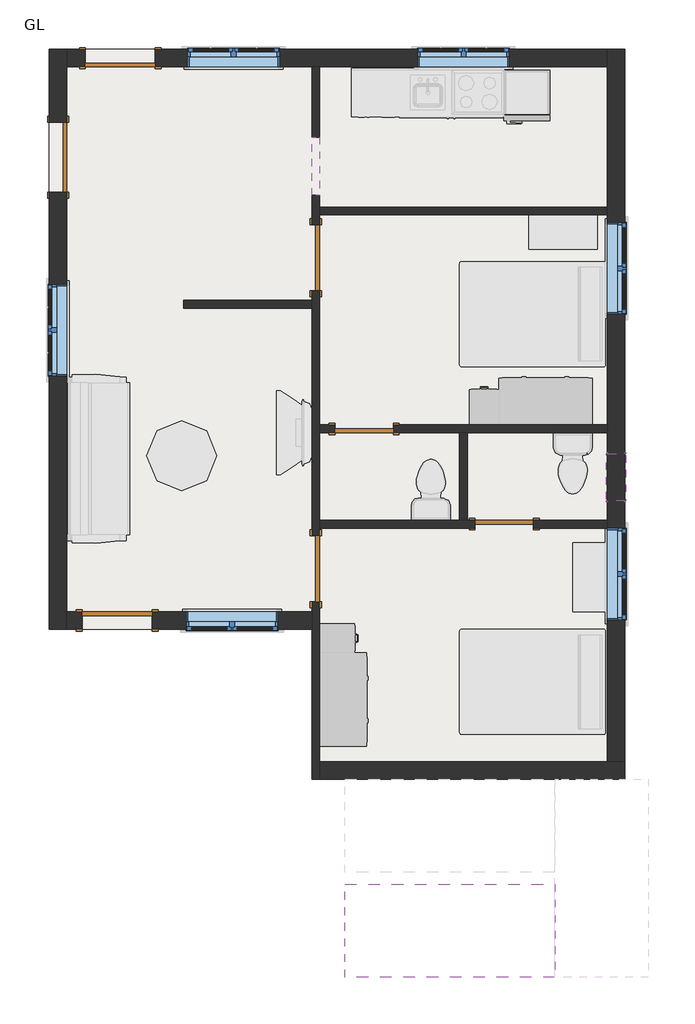
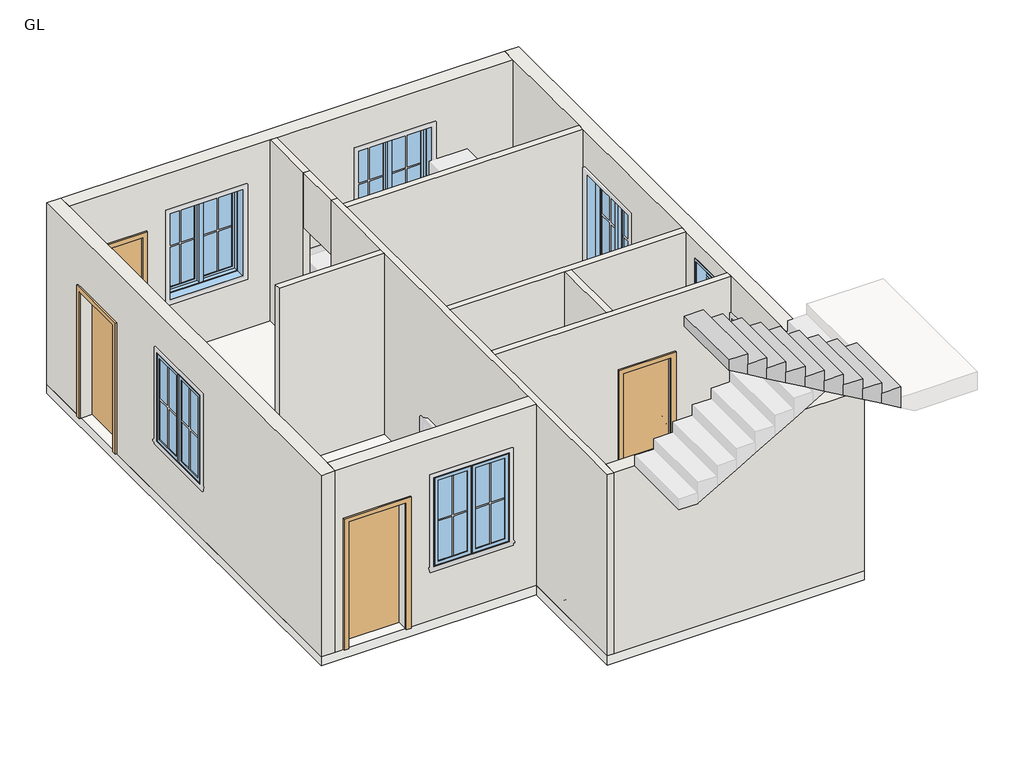
# One storey, part 1 of 2: 13 walls, 7 doors, 7 windows, 1 slab, 1 stair flight.
"""IFC4 building model written with IfcOpenShell, lengths in millimetres."""

from ifc_helpers import new_model, si_unit, frame, origin, origin_with_axes, place, context, project, spatial, polyline, outline, extrude, faceted_brep, transform, mapped, element, save
from components import m_single_flush_0762_x_2032mm_63ada305, m_single_flush_0762_x_2032mm_debabc81, m_single_flush_0864_x_2032mm_c62421c0, m_single_flush_0915_x_2134mm_43602619, m_single_flush_0915_x_2134mm_1ddf3370, m_window_casement_double_1200_x_1500mm_04159c99, window_f2d8fef0

model = new_model("IFC4")

# Units and contexts
model_context = context("Model", 3, world=origin())
ifc_project = project(units=[si_unit("LENGTHUNIT", "METRE", prefix="MILLI")], contexts=[model_context])

# Site, building, storey
site = spatial("IfcSite", under=ifc_project)
building = spatial("IfcBuilding", under=site)
storey = spatial("IfcBuildingStorey", under=building, Name="GL", Elevation=0.0)

# Doors
placement = place(None, origin())
m_single_flush_0762_x_2032mm_shape = m_single_flush_0762_x_2032mm_63ada305(model_context)
element("IfcDoor", 1, ObjectType="M_Single-Flush : 0762 x 2032mm", at=placement, inside=storey, context=model_context, shape_type="MappedRepresentation", body=[
    mapped(m_single_flush_0762_x_2032mm_shape, transform((2297.1455952, -1088.4648653, 0.0), x_axis=(-1.0, 0.0, 0.0), y_axis=(0.0, -1.0, 0.0), z_axis=(0.0, 0.0, 1.0))),
])
m_single_flush_0762_x_2032mm_2_shape = m_single_flush_0762_x_2032mm_debabc81(model_context)
element("IfcDoor", 2, ObjectType="M_Single-Flush : 0762 x 2032mm", at=placement, inside=storey, context=model_context, shape_type="MappedRepresentation", body=[
    mapped(m_single_flush_0762_x_2032mm_2_shape, transform((466.7455952, 156.1351347, 0.0), x_axis=(-1.0, 0.0, 0.0), y_axis=(0.0, -1.0, 0.0), z_axis=(0.0, 0.0, 1.0))),
])
m_single_flush_0864_x_2032mm_shape = m_single_flush_0864_x_2032mm_c62421c0(model_context)
element("IfcDoor", 3, ObjectType="M_Single-Flush : 0864 x 2032mm", at=placement, inside=storey, context=model_context, shape_type="MappedRepresentation", body=[
    mapped(m_single_flush_0864_x_2032mm_shape, transform((-165.0544048, 2391.3351347, 0.0), x_axis=(0.0, 1.0, 0.0), y_axis=(-1.0, 0.0, 0.0), z_axis=(0.0, 0.0, 1.0))),
])
element("IfcDoor", 4, ObjectType="M_Single-Flush : 0864 x 2032mm", at=placement, inside=storey, context=model_context, shape_type="MappedRepresentation", body=[
    mapped(m_single_flush_0864_x_2032mm_shape, transform((-165.0544048, -1671.2648653, 0.0), x_axis=(0.0, 1.0, 0.0), y_axis=(-1.0, 0.0, 0.0), z_axis=(0.0, 0.0, 1.0))),
])
m_single_flush_0915_x_2134mm_shape = m_single_flush_0915_x_2134mm_43602619(model_context)
element("IfcDoor", 5, ObjectType="M_Single-Flush : 0915 x 2134mm", at=placement, inside=storey, context=model_context, shape_type="MappedRepresentation", body=[
    mapped(m_single_flush_0915_x_2134mm_shape, transform((-2758.7544048, -2345.7648653, 0.0), x_axis=(-1.0, 0.0, 0.0), y_axis=(0.0, -1.0, 0.0), z_axis=(0.0, 0.0, 1.0))),
])
element("IfcDoor", 6, ObjectType="M_Single-Flush : 0915 x 2134mm", at=placement, inside=storey, context=model_context, shape_type="MappedRepresentation", body=[
    mapped(m_single_flush_0915_x_2134mm_shape, transform((-3530.5544048, 3703.0351347, 0.0), x_axis=(0.0, 1.0, 0.0), y_axis=(-1.0, 0.0, 0.0), z_axis=(0.0, 0.0, 1.0))),
])
m_single_flush_0915_x_2134mm_2_shape = m_single_flush_0915_x_2134mm_1ddf3370(model_context)
element("IfcDoor", 7, ObjectType="M_Single-Flush : 0915 x 2134mm", at=placement, inside=storey, context=model_context, shape_type="MappedRepresentation", body=[
    mapped(m_single_flush_0915_x_2134mm_2_shape, transform((-2718.7544048, 4994.8351347, 0.0), x_axis=(-1.0, 0.0, 0.0), y_axis=(0.0, -1.0, 0.0), z_axis=(0.0, 0.0, 1.0))),
])

# Slab
element("IfcSlab", 8, ObjectType="6\" floor", at=placement, inside=storey, context=model_context, shape_type="SweptSolid", body=[
    extrude(outline(polyline([(3873.5455952, 5109.1351347), (3873.5455952, -4415.8648653), (-215.8544048, -4415.8648653), (-215.8544048, -2460.0648653), (-3644.8544048, -2460.0648653), (-3644.8544048, 5109.1351347), (3873.5455952, 5109.1351347)])), frame((0.0, 0.0, -152.4), z_axis=(0.0, 0.0, 1.0), x_axis=(1.0, 0.0, 0.0)), (0.0, 0.0, 1.0), 152.4),
])

# Stair flight
element("IfcStairFlight", 9, ObjectType="150mm Depth", at=placement, inside=storey, context=model_context, shape_type="Brep", body=[
    faceted_brep([(2654.3455952, -7006.6648653, 4989.0947368), (2959.1455952, -7006.6648653, 4989.0947368), (2959.1455952, -5787.4648653, 4989.0947368), (2654.3455952, -5787.4648653, 4989.0947368), (2654.3455952, -7006.6648653, 4815.7697495), (2959.1455952, -7006.6648653, 4639.3065916), (2959.1455952, -7006.6648653, 4812.6315789), (2959.1455952, -5787.4648653, 4639.3065916), (2654.3455952, -5787.4648653, 4815.7697495), (2349.5455952, -7006.6648653, 5165.5578947), (2654.3455952, -7006.6648653, 5165.5578947), (2654.3455952, -5787.4648653, 5165.5578947), (2349.5455952, -5787.4648653, 5165.5578947), (2349.5455952, -7006.6648653, 4992.2329074), (2349.5455952, -5787.4648653, 4992.2329074), (2044.7455952, -7006.6648653, 5342.0210526), (2349.5455952, -7006.6648653, 5342.0210526), (2349.5455952, -5787.4648653, 5342.0210526), (2044.7455952, -5787.4648653, 5342.0210526), (2044.7455952, -7006.6648653, 5168.6960653), (2044.7455952, -5787.4648653, 5168.6960653), (1739.9455952, -7006.6648653, 5518.4842105), (2044.7455952, -7006.6648653, 5518.4842105), (2044.7455952, -5787.4648653, 5518.4842105), (1739.9455952, -5787.4648653, 5518.4842105), (1739.9455952, -7006.6648653, 5345.1592232), (1739.9455952, -5787.4648653, 5345.1592232), (1435.1455952, -7006.6648653, 5694.9473684), (1739.9455952, -7006.6648653, 5694.9473684), (1739.9455952, -5787.4648653, 5694.9473684), (1435.1455952, -5787.4648653, 5694.9473684), (1435.1455952, -7006.6648653, 5521.6223811), (1435.1455952, -5787.4648653, 5521.6223811), (1130.3455952, -7006.6648653, 5871.4105263), (1435.1455952, -7006.6648653, 5871.4105263), (1435.1455952, -5787.4648653, 5871.4105263), (1130.3455952, -5787.4648653, 5871.4105263), (1130.3455952, -7006.6648653, 5698.0855389), (1130.3455952, -5787.4648653, 5698.0855389), (825.5455952, -7006.6648653, 6047.8736842), (1130.3455952, -7006.6648653, 6047.8736842), (1130.3455952, -5787.4648653, 6047.8736842), (825.5455952, -5787.4648653, 6047.8736842), (825.5455952, -7006.6648653, 5874.5486968), (825.5455952, -5787.4648653, 5874.5486968), (520.7455952, -7006.6648653, 6224.3368421), (825.5455952, -7006.6648653, 6224.3368421), (825.5455952, -5787.4648653, 6224.3368421), (520.7455952, -5787.4648653, 6224.3368421), (520.7455952, -7006.6648653, 6051.0118547), (520.7455952, -5787.4648653, 6051.0118547), (215.9455952, -7006.6648653, 6400.8), (520.7455952, -7006.6648653, 6400.8), (520.7455952, -5787.4648653, 6400.8), (215.9455952, -5787.4648653, 6400.8), (215.9455952, -7006.6648653, 6227.4750126), (215.9455952, -5787.4648653, 6227.4750126)], [[[0, 1, 2, 3]], [[1, 0, 4, 5, 6]], [[2, 1, 6, 5, 7]], [[3, 2, 7, 8]], [[9, 10, 11, 12]], [[10, 9, 13, 4, 0]], [[11, 10, 0, 3]], [[12, 11, 3, 8, 14]], [[15, 16, 17, 18]], [[16, 15, 19, 13, 9]], [[17, 16, 9, 12]], [[18, 17, 12, 14, 20]], [[21, 22, 23, 24]], [[22, 21, 25, 19, 15]], [[23, 22, 15, 18]], [[24, 23, 18, 20, 26]], [[27, 28, 29, 30]], [[28, 27, 31, 25, 21]], [[29, 28, 21, 24]], [[30, 29, 24, 26, 32]], [[33, 34, 35, 36]], [[34, 33, 37, 31, 27]], [[35, 34, 27, 30]], [[36, 35, 30, 32, 38]], [[39, 40, 41, 42]], [[40, 39, 43, 37, 33]], [[41, 40, 33, 36]], [[42, 41, 36, 38, 44]], [[45, 46, 47, 48]], [[46, 45, 49, 43, 39]], [[47, 46, 39, 42]], [[48, 47, 42, 44, 50]], [[51, 52, 53, 54]], [[52, 51, 55, 49, 45]], [[53, 52, 45, 48]], [[54, 53, 48, 50, 56]], [[51, 54, 56, 55]], [[5, 4, 13, 19, 25, 31, 37, 43, 49, 55, 56, 50, 44, 38, 32, 26, 20, 14, 8, 7]]]),
])

# Walls
element("IfcWall", 10, ObjectType="4\" wall", at=placement, inside=storey, context=model_context, shape_type="Brep", body=[
    faceted_brep([(-215.8544048, 3204.1351347, 0.0), (-215.8544048, 2823.3351347, 0.0), (-215.8544048, 2823.3351347, 2032.0), (-215.8544048, 1959.3351347, 2032.0), (-215.8544048, 1959.3351347, 0.0), (-215.8544048, 1832.5351347, 0.0), (-215.8544048, 1730.9351347, 0.0), (-215.8544048, -1239.2648653, 0.0), (-215.8544048, -1239.2648653, 2032.0), (-215.8544048, -2103.2648653, 2032.0), (-215.8544048, -2103.2648653, 0.0), (-215.8544048, -2231.4648653, 0.0), (-215.8544048, -2460.0648653, 0.0), (-215.8544048, -4415.8648653, 0.0), (-215.8544048, -4415.8648653, 3048.0), (-215.8544048, -2460.0648653, 3048.0), (-215.8544048, -2231.4648653, 3048.0), (-215.8544048, 1730.9351347, 3048.0), (-215.8544048, 1832.5351347, 3048.0), (-215.8544048, 3204.1351347, 3048.0), (-215.8544048, 3204.1351347, 2133.6), (-114.2544048, 2823.3351347, 2032.0), (-114.2544048, 2823.3351347, 0.0), (-114.2544048, 2950.1351347, 0.0), (-114.2544048, 3051.7351347, 0.0), (-114.2544048, 3204.1351347, 0.0), (-114.2544048, 3204.1351347, 2133.6), (-114.2544048, 3204.1351347, 3048.0), (-114.2544048, 3051.7351347, 3048.0), (-114.2544048, 2950.1351347, 3048.0), (-114.2544048, 206.9351347, 3048.0), (-114.2544048, 105.3351347, 3048.0), (-114.2544048, -1037.6648653, 3048.0), (-114.2544048, -1139.2648653, 3048.0), (-114.2544048, -4187.2648653, 3048.0), (-114.2544048, -4415.8648653, 3048.0), (-114.2544048, -4415.8648653, 0.0), (-114.2544048, -4187.2648653, 0.0), (-114.2544048, -2103.2648653, 0.0), (-114.2544048, -2103.2648653, 2032.0), (-114.2544048, -1239.2648653, 2032.0), (-114.2544048, -1239.2648653, 0.0), (-114.2544048, -1139.2648653, 0.0), (-114.2544048, -1037.6648653, 0.0), (-114.2544048, 105.3351347, 0.0), (-114.2544048, 206.9351347, 0.0), (-114.2544048, 1959.3351347, 0.0), (-114.2544048, 1959.3351347, 2032.0)], [[[0, 1, 2, 3, 4, 5, 6, 7, 8, 9, 10, 11, 12, 13, 14, 15, 16, 17, 18, 19, 20]], [[21, 22, 23, 24, 25, 26, 27, 28, 29, 30, 31, 32, 33, 34, 35, 36, 37, 38, 39, 40, 41, 42, 43, 44, 45, 46, 47]], [[36, 13, 12, 11, 10, 38, 37]], [[25, 24, 23, 22, 1, 0]], [[46, 45, 44, 43, 42, 41, 7, 6, 5, 4]], [[19, 18, 17, 16, 15, 14, 35, 34, 33, 32, 31, 30, 29, 28, 27]], [[0, 20, 19, 27, 26, 25]], [[14, 13, 36, 35]], [[8, 40, 39, 9]], [[9, 39, 38, 10]], [[4, 3, 47, 46]], [[3, 2, 21, 47]], [[2, 1, 22, 21]], [[40, 8, 7, 41]]]),
])
element("IfcWall", 11, ObjectType="4\" wall", at=placement, inside=storey, context=model_context, shape_type="Brep", body=[
    faceted_brep([(-114.2544048, -1139.2648653, 0.0), (1916.1455952, -1139.2648653, 0.0), (1916.1455952, -1139.2648653, 2032.0), (2678.1455952, -1139.2648653, 2032.0), (2678.1455952, -1139.2648653, 0.0), (3644.9455952, -1139.2648653, 0.0), (3644.9455952, -1139.2648653, 900.0), (3644.9455952, -1139.2648653, 2400.0), (3644.9455952, -1139.2648653, 3048.0), (-114.2544048, -1139.2648653, 3048.0), (1916.1455952, -1037.6648653, 2032.0), (1916.1455952, -1037.6648653, 0.0), (1816.1455952, -1037.6648653, 0.0), (1714.5455952, -1037.6648653, 0.0), (-114.2544048, -1037.6648653, 0.0), (-114.2544048, -1037.6648653, 3048.0), (1714.5455952, -1037.6648653, 3048.0), (1816.1455952, -1037.6648653, 3048.0), (3644.9455952, -1037.6648653, 3048.0), (3644.9455952, -1037.6648653, 0.0), (2678.1455952, -1037.6648653, 0.0), (2678.1455952, -1037.6648653, 2032.0)], [[[0, 1, 2, 3, 4, 5, 6, 7, 8, 9]], [[10, 11, 12, 13, 14, 15, 16, 17, 18, 19, 20, 21]], [[20, 19, 5, 4]], [[14, 13, 12, 11, 1, 0]], [[9, 8, 18, 17, 16, 15]], [[8, 7, 6, 5, 19, 18]], [[0, 9, 15, 14]], [[2, 1, 11, 10]], [[3, 2, 10, 21]], [[4, 3, 21, 20]]]),
])
element("IfcWall", 12, ObjectType="4\" wall", at=placement, inside=storey, context=model_context, shape_type="Brep", body=[
    faceted_brep([(85.7455952, 206.9351347, 2032.0), (85.7455952, 206.9351347, 0.0), (-114.2544048, 206.9351347, 0.0), (-114.2544048, 206.9351347, 3048.0), (3644.9455952, 206.9351347, 3048.0), (3644.9455952, 206.9351347, 0.0), (847.7455952, 206.9351347, 0.0), (847.7455952, 206.9351347, 2032.0), (-114.2544048, 105.3351347, 0.0), (85.7455952, 105.3351347, 0.0), (85.7455952, 105.3351347, 2032.0), (847.7455952, 105.3351347, 2032.0), (847.7455952, 105.3351347, 0.0), (1714.5455952, 105.3351347, 0.0), (1816.1455952, 105.3351347, 0.0), (3644.9455952, 105.3351347, 0.0), (3644.9455952, 105.3351347, 3048.0), (1816.1455952, 105.3351347, 3048.0), (1714.5455952, 105.3351347, 3048.0), (-114.2544048, 105.3351347, 3048.0)], [[[0, 1, 2, 3, 4, 5, 6, 7]], [[8, 9, 10, 11, 12, 13, 14, 15, 16, 17, 18, 19]], [[6, 5, 15, 14, 13, 12]], [[2, 1, 9, 8]], [[4, 3, 19, 18, 17, 16]], [[5, 4, 16, 15]], [[3, 2, 8, 19]], [[10, 9, 1, 0]], [[11, 10, 0, 7]], [[12, 11, 7, 6]]]),
])
element("IfcWall", 13, ObjectType="4\" wall", at=placement, inside=storey, context=model_context, shape_type="SweptSolid", body=[
    extrude(outline(polyline([(-215.8544048, 1730.9351347), (-1892.2544048, 1730.9351347), (-1892.2544048, 1832.5351347), (-215.8544048, 1832.5351347), (-215.8544048, 1730.9351347)])), origin_with_axes(), (0.0, 0.0, 1.0), 3048.0),
])
element("IfcWall", 14, ObjectType="4\" wall", at=placement, inside=storey, context=model_context, shape_type="SweptSolid", body=[
    extrude(outline(polyline([(-114.2544048, 3051.7351347), (3644.9455952, 3051.7351347), (3644.9455952, 2950.1351347), (-114.2544048, 2950.1351347), (-114.2544048, 3051.7351347)])), origin_with_axes(), (0.0, 0.0, 1.0), 3048.0),
])
element("IfcWall", 15, ObjectType="4\" wall", at=placement, inside=storey, context=model_context, shape_type="SweptSolid", body=[
    extrude(outline(polyline([(1714.5455952, -1037.6648653), (1714.5455952, 105.3351347), (1816.1455952, 105.3351347), (1816.1455952, -1037.6648653), (1714.5455952, -1037.6648653)])), origin_with_axes(), (0.0, 0.0, 1.0), 3048.0),
])
element("IfcWall", 16, ObjectType="4\" wall", at=placement, inside=storey, context=model_context, shape_type="Brep", body=[
    faceted_brep([(-215.8544048, 4880.5351347, 0.0), (-215.8544048, 3966.1351347, 0.0), (-215.8544048, 3966.1351347, 2133.6), (-215.8544048, 3966.1351347, 3048.0), (-215.8544048, 4880.5351347, 3048.0), (-114.2544048, 4880.5351347, 0.0), (-114.2544048, 4880.5351347, 3048.0), (-114.2544048, 3966.1351347, 3048.0), (-114.2544048, 3966.1351347, 2133.6), (-114.2544048, 3966.1351347, 0.0)], [[[0, 1, 2, 3, 4]], [[5, 6, 7, 8, 9]], [[1, 0, 5, 9]], [[3, 2, 1, 9, 8, 7]], [[4, 3, 7, 6]], [[0, 4, 6, 5]]]),
])
element("IfcWall", 17, ObjectType="4\" wall", at=placement, inside=storey, context=model_context, shape_type="SweptSolid", body=[
    extrude(outline(polyline([(-215.8544048, 3204.1351347), (-215.8544048, 3966.1351347), (-114.2544048, 3966.1351347), (-114.2544048, 3204.1351347), (-215.8544048, 3204.1351347)])), frame((0.0, 0.0, 2133.6), z_axis=(0.0, 0.0, 1.0), x_axis=(1.0, 0.0, 0.0)), (0.0, 0.0, 1.0), 914.4),
])
element("IfcWall", 18, ObjectType="9\" wall", at=placement, inside=storey, context=model_context, shape_type="Brep", body=[
    faceted_brep([(-3644.8544048, 5109.1351347, 0.0), (-3644.8544048, 4160.5351347, 0.0), (-3644.8544048, 4160.5351347, 2134.0), (-3644.8544048, 3245.5351347, 2134.0), (-3644.8544048, 3245.5351347, 0.0), (-3644.8544048, -2460.0648653, 0.0), (-3644.8544048, -2460.0648653, 3048.0), (-3644.8544048, 5109.1351347, 3048.0), (-3644.8544048, 2045.5351347, 2400.0), (-3644.8544048, 845.5351347, 2400.0), (-3644.8544048, 845.5351347, 900.0), (-3644.8544048, 2045.5351347, 900.0), (-3416.2544048, 4160.5351347, 2134.0), (-3416.2544048, 4160.5351347, 0.0), (-3416.2544048, 4880.5351347, 0.0), (-3416.2544048, 5109.1351347, 0.0), (-3416.2544048, 5109.1351347, 3048.0), (-3416.2544048, 4880.5351347, 3048.0), (-3416.2544048, -2231.4648653, 3048.0), (-3416.2544048, -2460.0648653, 3048.0), (-3416.2544048, -2460.0648653, 0.0), (-3416.2544048, -2231.4648653, 0.0), (-3416.2544048, 3245.5351347, 0.0), (-3416.2544048, 3245.5351347, 2134.0), (-3416.2544048, 2045.5351347, 2400.0), (-3416.2544048, 2045.5351347, 900.0), (-3416.2544048, 845.5351347, 900.0), (-3416.2544048, 845.5351347, 2400.0)], [[[0, 1, 2, 3, 4, 5, 6, 7], [8, 9, 10, 11]], [[12, 13, 14, 15, 16, 17, 18, 19, 20, 21, 22, 23], [24, 25, 26, 27]], [[15, 14, 13, 1, 0]], [[22, 21, 20, 5, 4]], [[7, 6, 19, 18, 17, 16]], [[6, 5, 20, 19]], [[0, 7, 16, 15]], [[2, 1, 13, 12]], [[3, 2, 12, 23]], [[4, 3, 23, 22]], [[25, 24, 8, 11]], [[26, 25, 11, 10]], [[27, 26, 10, 9]], [[24, 27, 9, 8]]]),
])
element("IfcWall", 19, ObjectType="9\" wall", at=placement, inside=storey, context=model_context, shape_type="SweptSolid", body=[
    extrude(outline(polyline([(0.0, -3416.2544048), (0.0, -3216.2544048), (2134.0, -3216.2544048), (2134.0, -2301.2544048), (0.0, -2301.2544048), (0.0, -215.8544048), (3048.0, -215.8544048), (3048.0, -3416.2544048), (0.0, -3416.2544048)]), holes=[polyline([(2400.0, -1858.5544048), (2400.0, -658.5544048), (900.0, -658.5544048), (900.0, -1858.5544048), (2400.0, -1858.5544048)])]), frame((0.0, -2460.0648653, 0.0), z_axis=(0.0, 1.0, 0.0), x_axis=(0.0, 0.0, 1.0)), (0.0, 0.0, 1.0), 228.6),
])
element("IfcWall", 20, ObjectType="9\" wall", at=placement, inside=storey, context=model_context, shape_type="Brep", body=[
    faceted_brep([(-114.2544048, -4415.8648653, 0.0), (3873.5455952, -4415.8648653, 0.0), (3873.5455952, -4415.8648653, 3048.0), (-114.2544048, -4415.8648653, 3048.0), (-114.2544048, -4187.2648653, 0.0), (-114.2544048, -4187.2648653, 3048.0), (3644.9455952, -4187.2648653, 3048.0), (3873.5455952, -4187.2648653, 3048.0), (3873.5455952, -4187.2648653, 0.0), (3644.9455952, -4187.2648653, 0.0)], [[[0, 1, 2, 3]], [[4, 5, 6, 7, 8, 9]], [[1, 0, 4, 9, 8]], [[3, 2, 7, 6, 5]], [[0, 3, 5, 4]], [[2, 1, 8, 7]]]),
])
element("IfcWall", 21, ObjectType="9\" wall", at=placement, inside=storey, context=model_context, shape_type="Brep", body=[
    faceted_brep([(3873.5455952, -4187.2648653, 0.0), (3873.5455952, 5109.1351347, 0.0), (3873.5455952, 5109.1351347, 3048.0), (3873.5455952, -4187.2648653, 3048.0), (3873.5455952, 1650.1351347, 2400.0), (3873.5455952, 2850.1351347, 2400.0), (3873.5455952, 2850.1351347, 900.0), (3873.5455952, 1650.1351347, 900.0), (3873.5455952, -2339.2648653, 2400.0), (3873.5455952, -1139.2648653, 2400.0), (3873.5455952, -1139.2648653, 900.0), (3873.5455952, -2339.2648653, 900.0), (3873.5455952, -170.8898653, 2743.2), (3873.5455952, -170.8898653, 2133.6), (3873.5455952, -780.4898653, 2133.6), (3873.5455952, -780.4898653, 2743.2), (3644.9455952, -4187.2648653, 0.0), (3644.9455952, -4187.2648653, 3048.0), (3644.9455952, -1139.2648653, 3048.0), (3644.9455952, -1037.6648653, 3048.0), (3644.9455952, 105.3351347, 3048.0), (3644.9455952, 206.9351347, 3048.0), (3644.9455952, 2950.1351347, 3048.0), (3644.9455952, 3051.7351347, 3048.0), (3644.9455952, 4880.5351347, 3048.0), (3644.9455952, 5109.1351347, 3048.0), (3644.9455952, 5109.1351347, 0.0), (3644.9455952, 4880.5351347, 0.0), (3644.9455952, 3051.7351347, 0.0), (3644.9455952, 2950.1351347, 0.0), (3644.9455952, 206.9351347, 0.0), (3644.9455952, 105.3351347, 0.0), (3644.9455952, -1037.6648653, 0.0), (3644.9455952, -1139.2648653, 0.0), (3644.9455952, 1650.1351347, 2400.0), (3644.9455952, 1650.1351347, 900.0), (3644.9455952, 2850.1351347, 900.0), (3644.9455952, 2850.1351347, 2400.0), (3644.9455952, -2339.2648653, 2400.0), (3644.9455952, -2339.2648653, 900.0), (3644.9455952, -1139.2648653, 900.0), (3644.9455952, -1139.2648653, 2400.0), (3644.9455952, -170.8898653, 2743.2), (3644.9455952, -780.4898653, 2743.2), (3644.9455952, -780.4898653, 2133.6), (3644.9455952, -170.8898653, 2133.6)], [[[0, 1, 2, 3], [4, 5, 6, 7], [8, 9, 10, 11], [12, 13, 14, 15]], [[16, 17, 18, 19, 20, 21, 22, 23, 24, 25, 26, 27, 28, 29, 30, 31, 32, 33], [34, 35, 36, 37], [38, 39, 40, 41], [42, 43, 44, 45]], [[1, 0, 16, 33, 32, 31, 30, 29, 28, 27, 26]], [[3, 2, 25, 24, 23, 22, 21, 20, 19, 18, 17]], [[0, 3, 17, 16]], [[2, 1, 26, 25]], [[35, 34, 4, 7]], [[36, 35, 7, 6]], [[37, 36, 6, 5]], [[34, 37, 5, 4]], [[39, 38, 8, 11]], [[40, 39, 11, 10]], [[41, 40, 10, 9]], [[38, 41, 9, 8]], [[13, 12, 42, 45]], [[14, 13, 45, 44]], [[15, 14, 44, 43]], [[12, 15, 43, 42]]]),
])
element("IfcWall", 22, ObjectType="9\" wall", at=placement, inside=storey, context=model_context, shape_type="Brep", body=[
    faceted_brep([(-3176.2544048, 5109.1351347, 2134.0), (-3176.2544048, 5109.1351347, 0.0), (-3416.2544048, 5109.1351347, 0.0), (-3416.2544048, 5109.1351347, 3048.0), (3644.9455952, 5109.1351347, 3048.0), (3644.9455952, 5109.1351347, 0.0), (-2261.2544048, 5109.1351347, 0.0), (-2261.2544048, 5109.1351347, 2134.0), (2365.3455952, 5109.1351347, 2400.0), (1165.3455952, 5109.1351347, 2400.0), (1165.3455952, 5109.1351347, 900.0), (2365.3455952, 5109.1351347, 900.0), (-638.5544048, 5109.1351347, 2400.0), (-1838.5544048, 5109.1351347, 2400.0), (-1838.5544048, 5109.1351347, 900.0), (-638.5544048, 5109.1351347, 900.0), (-3416.2544048, 4880.5351347, 0.0), (-3176.2544048, 4880.5351347, 0.0), (-3176.2544048, 4880.5351347, 2134.0), (-2261.2544048, 4880.5351347, 2134.0), (-2261.2544048, 4880.5351347, 0.0), (-215.8544048, 4880.5351347, 0.0), (-114.2544048, 4880.5351347, 0.0), (3644.9455952, 4880.5351347, 0.0), (3644.9455952, 4880.5351347, 3048.0), (-114.2544048, 4880.5351347, 3048.0), (-215.8544048, 4880.5351347, 3048.0), (-3416.2544048, 4880.5351347, 3048.0), (2365.3455952, 4880.5351347, 2400.0), (2365.3455952, 4880.5351347, 900.0), (1165.3455952, 4880.5351347, 900.0), (1165.3455952, 4880.5351347, 2400.0), (-638.5544048, 4880.5351347, 2400.0), (-638.5544048, 4880.5351347, 900.0), (-1838.5544048, 4880.5351347, 900.0), (-1838.5544048, 4880.5351347, 2400.0)], [[[0, 1, 2, 3, 4, 5, 6, 7], [8, 9, 10, 11], [12, 13, 14, 15]], [[16, 17, 18, 19, 20, 21, 22, 23, 24, 25, 26, 27], [28, 29, 30, 31], [32, 33, 34, 35]], [[6, 5, 23, 22, 21, 20]], [[2, 1, 17, 16]], [[4, 3, 27, 26, 25, 24]], [[5, 4, 24, 23]], [[3, 2, 16, 27]], [[18, 17, 1, 0]], [[19, 18, 0, 7]], [[20, 19, 7, 6]], [[29, 28, 8, 11]], [[30, 29, 11, 10]], [[31, 30, 10, 9]], [[28, 31, 9, 8]], [[33, 32, 12, 15]], [[34, 33, 15, 14]], [[35, 34, 14, 13]], [[32, 35, 13, 12]]]),
])

# Windows
m_window_casement_double_1200_x_1500mm_shape = m_window_casement_double_1200_x_1500mm_04159c99(model_context)
element("IfcWindow", 23, ObjectType="M_Window-Casement-Double : 1200 x 1500mm", at=placement, inside=storey, context=model_context, shape_type="MappedRepresentation", body=[
    mapped(m_window_casement_double_1200_x_1500mm_shape, transform((1765.3455952, 4994.8351347, 0.0), x_axis=(1.0, 0.0, 0.0), y_axis=(0.0, 1.0, 0.0), z_axis=(0.0, 0.0, 1.0))),
])
element("IfcWindow", 24, ObjectType="M_Window-Casement-Double : 1200 x 1500mm", at=placement, inside=storey, context=model_context, shape_type="MappedRepresentation", body=[
    mapped(m_window_casement_double_1200_x_1500mm_shape, transform((3759.2455952, 2250.1351347, 0.0), x_axis=(0.0, -1.0, 0.0), y_axis=(1.0, 0.0, 0.0), z_axis=(0.0, 0.0, 1.0))),
])
element("IfcWindow", 25, ObjectType="M_Window-Casement-Double : 1200 x 1500mm", at=placement, inside=storey, context=model_context, shape_type="MappedRepresentation", body=[
    mapped(m_window_casement_double_1200_x_1500mm_shape, transform((3759.2455952, -1739.2648653, 0.0), x_axis=(0.0, -1.0, 0.0), y_axis=(1.0, 0.0, 0.0), z_axis=(0.0, 0.0, 1.0))),
])
element("IfcWindow", 26, ObjectType="M_Window-Casement-Double : 1200 x 1500mm", at=placement, inside=storey, context=model_context, shape_type="MappedRepresentation", body=[
    mapped(m_window_casement_double_1200_x_1500mm_shape, transform((-1258.5544048, -2345.7648653, 0.0), x_axis=(-1.0, 0.0, 0.0), y_axis=(0.0, -1.0, 0.0), z_axis=(0.0, 0.0, 1.0))),
])
element("IfcWindow", 27, ObjectType="M_Window-Casement-Double : 1200 x 1500mm", at=placement, inside=storey, context=model_context, shape_type="MappedRepresentation", body=[
    mapped(m_window_casement_double_1200_x_1500mm_shape, transform((-3530.5544048, 1445.5351347, 0.0), x_axis=(0.0, 1.0, 0.0), y_axis=(-1.0, 0.0, 0.0), z_axis=(0.0, 0.0, 1.0))),
])
element("IfcWindow", 28, ObjectType="M_Window-Casement-Double : 1200 x 1500mm", at=placement, inside=storey, context=model_context, shape_type="MappedRepresentation", body=[
    mapped(m_window_casement_double_1200_x_1500mm_shape, transform((-1238.5544048, 4994.8351347, 0.0), x_axis=(1.0, 0.0, 0.0), y_axis=(0.0, 1.0, 0.0), z_axis=(0.0, 0.0, 1.0))),
])
window_shape = window_f2d8fef0(model_context)
element("IfcWindow", 29, ObjectType="Window-Louvers : 24\" x 24\"", at=placement, inside=storey, context=model_context, shape_type="MappedRepresentation", body=[
    mapped(window_shape, transform((3765.5955952, -475.6898653, 1219.2), x_axis=(0.0, -1.0, 0.0), y_axis=(1.0, 0.0, 0.0), z_axis=(0.0, 0.0, 1.0))),
])

save(model, "model.ifc")

# Revit data of these elements
# Type "M_Single-Flush : 0762 x 2032mm"
#   Type Mark = "28"
#   Construction Type Id = "MDOOR"
#   Analytic Construction = "Metal"
#   Thickness = 0.167323 ft
#   Thermal Resistance (R) = 0.270117 (m²·K)/W
#   Heat Transfer Coefficient (U) = 3.7021 W/(m²·K)
#   Height = 6.666667 ft
#   Trim Projection Ext = 0.082021 ft
#   Trim Projection Int = 0.082021 ft
#   Trim Width = 0.249344 ft
#   Width = 2.5 ft
#   Define Thermal Properties by = 1
#   Define Thermal Properties by = 1
#   Door Material = Door - Panel
#   Frame Material = Door - Frame
#   Visual Light Transmittance = 0
#   Solar Heat Gain Coefficient = 0
#   Function = (empty or 0)
#   Wall Closure = (empty or 0)
# Type "M_Single-Flush : 0864 x 2032mm"
#   Type Mark = "32"
#   Construction Type Id = "MDOOR"
#   Analytic Construction = "Metal"
#   Thickness = 0.167323 ft
#   Thermal Resistance (R) = 0.270117 (m²·K)/W
#   Heat Transfer Coefficient (U) = 3.7021 W/(m²·K)
#   Height = 6.666667 ft
#   Trim Projection Ext = 0.082021 ft
#   Trim Projection Int = 0.082021 ft
#   Trim Width = 0.249344 ft
#   Width = 2.834646 ft
#   Define Thermal Properties by = 1
#   Define Thermal Properties by = 1
#   Door Material = Door - Panel
#   Frame Material = Door - Frame
#   Visual Light Transmittance = 0
#   Solar Heat Gain Coefficient = 0
#   Function = (empty or 0)
#   Wall Closure = (empty or 0)
# Type "M_Single-Flush : 0915 x 2134mm"
#   Type Mark = "20"
#   Construction Type Id = "MDOOR"
#   Analytic Construction = "Metal"
#   Thickness = 0.167323 ft
#   Thermal Resistance (R) = 0.270117 (m²·K)/W
#   Heat Transfer Coefficient (U) = 3.7021 W/(m²·K)
#   Height = 7.001312 ft
#   Trim Projection Ext = 0.082021 ft
#   Trim Projection Int = 0.082021 ft
#   Trim Width = 0.249344 ft
#   Width = 3.001969 ft
#   Define Thermal Properties by = 1
#   Define Thermal Properties by = 1
#   Door Material = Door - Panel
#   Frame Material = Door - Frame
#   Visual Light Transmittance = 0
#   Solar Heat Gain Coefficient = 0
#   Function = (empty or 0)
#   Wall Closure = (empty or 0)
# Type "6\" floor"
#   Function = 0
#   Layers, outside or top first: 0.5 ft no material (function 1)
# Type "4\" wall"
#   Layers, outside or top first: 0.333333 ft no material (function 1)
# Type "9\" wall"
#   Layers, outside or top first: 0.75 ft no material (function 1)
# Type "M_Window-Casement-Double : 1200 x 1500mm"
#   Type Mark = "25"
#   Fire Rating = "0.5h"
#   Assembly Code = "B2020100"
#   Analytic Construction = "Double glazing - domestic"
#   Frame Extension [instance default] = 0.020833 ft
#   Window Inset [instance default] = 0.0 ft
#   Wall Thickness [instance default] = 0.492126 ft
#   Interior Wall Closure [instance default] = 0.179626 ft
#   Half Width = 1.968504 ft
#   Visual Light Transmittance = 0.81
#   Thermal Resistance (R) = 0.319569 (m²·K)/W
#   Solar Heat Gain Coefficient = 0.76
#   Rough Width = 3.98622 ft
#   Rough Height = 4.970472 ft
#   Height = 4.92126 ft
#   Heat Transfer Coefficient (U) = 3.12929 W/(m²·K)
#   Exterior Wall Closure [instance default] = 0.104331 ft
#   Extension Jamb [instance default] = 0.179626 ft
#   Default Sill Height = 2.952756 ft
#   Width = 3.937008 ft
#   Define Thermal Properties by = 0
#   Muntin Visibility = yes
#   Interior Trim Visibility [instance default] = yes
#   Exterior Trim Visibility [instance default] = yes
#   Extension Jamb Visibility [instance default] = yes
#   Interior Trim Material = Wood - Stained
#   Muntin Pattern = M_Muntin Pattern_2x2 : M_Muntin Pattern_2x2
#   Interior Trim = M_Trim-Window-Interior-Flat : Picture Frame
#   Interior Frame Material = Wood - Stained
#   Glass Panel Material = Glass
#   Exterior Trim Material = Clad - White
#   Exterior Trim = M_Trim-Window-Exterior-Flat : with Sill
#   Exterior Frame Material = Clad - White
#   Wall Closure = (empty or 0)
# Type "Window-Louvers : 24\" x 24\""
#   Type Mark = "28"
#   Construction Type Id = "GSP4R"
#   Assembly Code = "B20"
#   Analytic Construction = "1/8 in Pilkington single glazing"
#   Visual Light Transmittance = 0.9
#   Thermal Resistance (R) = 0.271106 (m²·K)/W
#   Solar Heat Gain Coefficient = 0.78
#   Max Height = 1.978553 ft
#   Height = 2.0 ft
#   Heat Transfer Coefficient (U) = 3.6886 W/(m²·K)
#   Blade Width [instance default] = 1.875 ft
#   Blade Vertical Thickness = 0.029463 ft
#   Blade Thickness = 0.020833 ft
#   Blade Spacing = 0.125 ft
#   Blade Height = 0.154463 ft
#   Blade Depth = 0.25 ft
#   Blade Angle = 45.00°
#   Default Sill Height = 3.0 ft
#   Trim Projection_Exterior = 0.041667 ft
#   Trim Projection_Interior = 0.041667 ft
#   Trim Width_Exterior = 0.125 ft
#   Trim Width_Interior = 0.125 ft
#   Width = 2.0 ft
#   Max Blade Count = 12
#   Define Thermal Properties by = 1
#   Blade Count = 12
#   Frame Material = Birch
#   Louver Material = Birch
#   Trim Exterior Material = Birch
#   Trim Interior Material = Birch
#   Wall Closure = (empty or 0)
# Elements 1, 2 (IfcDoor, "M_Single-Flush : 0762 x 2032mm")
#   Phase Created = New Construction
#   Materials on its faces: "Door - Frame", "Door - Panel"
# Elements 3, 4 (IfcDoor, "M_Single-Flush : 0864 x 2032mm")
#   Phase Created = New Construction
#   Materials on its faces: "Door - Frame", "Door - Panel"
# Elements 5, 6, 7 (IfcDoor, "M_Single-Flush : 0915 x 2134mm")
#   Phase Created = New Construction
#   Materials on its faces: "Door - Frame", "Door - Panel"
# Element 8 (IfcSlab, "6\" floor")
#   Height Offset From Level = 0.0 ft
#   Phase Created = New Construction
#   Materials on its faces: "Default Floor"
# Element 9 (IfcStairFlight, "150mm Depth")
#   Phase Created = New Construction
#   Materials on its faces: "Concrete, Cast In Situ"
# Elements 10, 11, 12, 13, 14, 15, 16 (IfcWall, "4\" wall")
#   Top Offset = 0.0 ft
#   Base Offset = 0.0 ft
#   Unconnected Height = 10.0 ft
#   wall height = 10.0 ft
#   Phase Created = New Construction
#   Base Constraint = GL
#   Materials on its faces: "Default Wall"
# Element 17 (IfcWall, "4\" wall")
#   built-in parameter 1001111 = 7.0 ft
#   Top Offset = 0.0 ft
#   Base Offset = 7.0 ft
#   Unconnected Height = 3.0 ft
#   wall height = 3.0 ft
#   Phase Created = New Construction
#   Base Constraint = GL
#   Materials on its faces: "Default Wall"
# Elements 18, 19, 20, 21, 22 (IfcWall, "9\" wall")
#   Top Offset = 0.0 ft
#   Base Offset = 0.0 ft
#   Unconnected Height = 10.0 ft
#   wall height = 10.0 ft
#   Phase Created = New Construction
#   Base Constraint = GL
#   Materials on its faces: "Default Wall"
# Element 23 (IfcWindow, "M_Window-Casement-Double : 1200 x 1500mm")
#   Mark = "1"
#   Window Inset = 0.0 ft
#   Interior Wall Closure = 0.179626 ft
#   Frame Extension = 0.020833 ft
#   Exterior Wall Closure = 0.104331 ft
#   Interior Trim Visibility = yes
#   Exterior Trim Visibility = yes
#   Phase Created = New Construction
#   Materials on its faces: "Wood - Stained", "Glass", "Clad - White"
# Element 24 (IfcWindow, "M_Window-Casement-Double : 1200 x 1500mm")
#   Mark = "2"
#   Window Inset = 0.0 ft
#   Interior Wall Closure = 0.179626 ft
#   Frame Extension = 0.020833 ft
#   Exterior Wall Closure = 0.104331 ft
#   Interior Trim Visibility = yes
#   Exterior Trim Visibility = yes
#   Phase Created = New Construction
#   Materials on its faces: "Wood - Stained", "Glass", "Clad - White"
# Element 25 (IfcWindow, "M_Window-Casement-Double : 1200 x 1500mm")
#   Mark = "3"
#   Window Inset = 0.0 ft
#   Interior Wall Closure = 0.179626 ft
#   Frame Extension = 0.020833 ft
#   Exterior Wall Closure = 0.104331 ft
#   Interior Trim Visibility = yes
#   Exterior Trim Visibility = yes
#   Phase Created = New Construction
#   Materials on its faces: "Wood - Stained", "Glass", "Clad - White"
# Element 26 (IfcWindow, "M_Window-Casement-Double : 1200 x 1500mm")
#   Mark = "4"
#   Window Inset = 0.0 ft
#   Interior Wall Closure = 0.179626 ft
#   Frame Extension = 0.020833 ft
#   Exterior Wall Closure = 0.104331 ft
#   Interior Trim Visibility = yes
#   Exterior Trim Visibility = yes
#   Phase Created = New Construction
#   Materials on its faces: "Wood - Stained", "Glass", "Clad - White"
# Element 27 (IfcWindow, "M_Window-Casement-Double : 1200 x 1500mm")
#   Mark = "5"
#   Window Inset = 0.0 ft
#   Interior Wall Closure = 0.179626 ft
#   Frame Extension = 0.020833 ft
#   Exterior Wall Closure = 0.104331 ft
#   Interior Trim Visibility = yes
#   Exterior Trim Visibility = yes
#   Phase Created = New Construction
#   Materials on its faces: "Wood - Stained", "Glass", "Clad - White"
# Element 28 (IfcWindow, "M_Window-Casement-Double : 1200 x 1500mm")
#   Mark = "6"
#   Window Inset = 0.0 ft
#   Interior Wall Closure = 0.179626 ft
#   Frame Extension = 0.020833 ft
#   Exterior Wall Closure = 0.104331 ft
#   Interior Trim Visibility = yes
#   Exterior Trim Visibility = yes
#   Phase Created = New Construction
#   Materials on its faces: "Wood - Stained", "Glass", "Clad - White"
# Element 29 (IfcWindow, "Window-Louvers : 24\" x 24\"")
#   Mark = "7"
#   Blade Width = 1.875 ft
#   Phase Created = New Construction
#   Materials on its faces: "Birch"
# Materials
#   "Door - Panel": class "Wood", colour RGB 210 159 95, transparency 0, Cost = 0
#   "Door - Frame": colour RGB 118 70 51, transparency 0, Cost = 0
#   "Wood - Stained": class "Wood", colour RGB 224 178 126, transparency 0, Cost = 0
#   "Glass": class "Glass", colour RGB 0 128 192, transparency 0.9, Description = "Soda Lime Glass", Cost = 0
#   "Clad - White": class "Wood", colour RGB 242 242 238, transparency 0, Cost = 0
#   "Birch": class "Wood", colour RGB 224 178 126, transparency 0, Description = "Betula Alleghaniensis", Cost = 0
#   "Default Floor": colour RGB 127 127 127, transparency 0, Cost = 0
#   "Concrete, Cast In Situ": class "Concrete", colour RGB 192 192 192, transparency 0, Description = "physical material", Cost = 0
#   "Default Wall": colour RGB 128 128 128, transparency 0, Cost = 0
